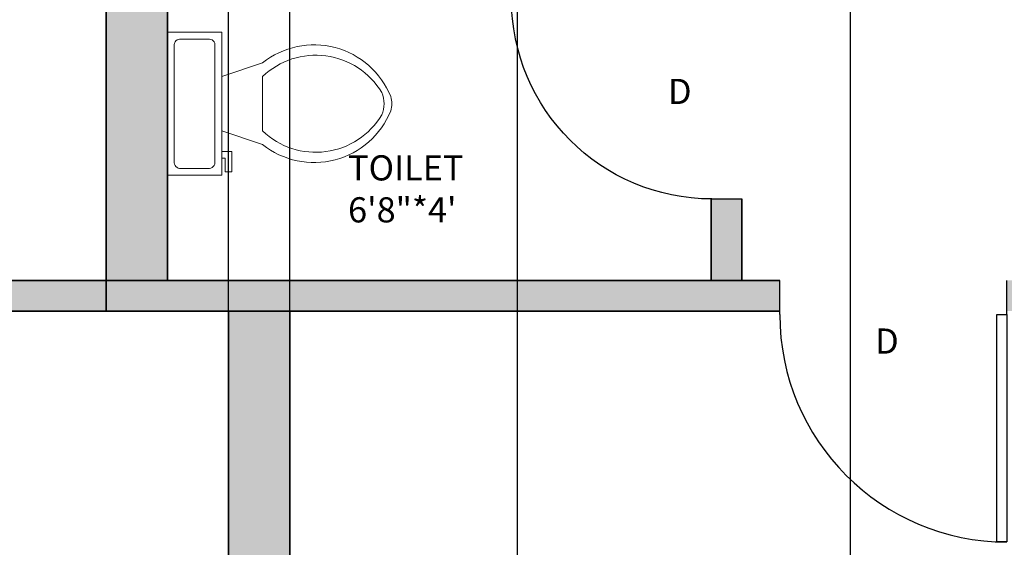
# Model space of a CAD drawing. Units: inches. Extents: x 1998 to 2588, y 1139 to 1977.
# Tile 24 of 134: x 2075 to 2220, y 1668 to 1746. Entities that reach past the tile are written whole.
import ezdxf

# ---------------------------------------------------------------- set-up
doc = ezdxf.new("R2010")
doc.units = ezdxf.units.IN
for name, color, linetype, lineweight in [('A-ANNO-DIMS', 2, 'Continuous', 18), ('A-AREA-IDEN', 7, 'Continuous', 18), ('A-DOOR-IDEN', 7, 'Continuous', 18), ('A-FLOR-FIXT', 9, 'Continuous', 18), ('A-WALL-PATT', 252, 'Continuous', 13), ('DOOR', 52, 'Continuous', 25), ('WALL', 200, 'Continuous', 35)]:
    doc.layers.add(name, color=color, linetype=linetype, lineweight=lineweight)
doc.styles.get("Standard").update_dxf_attribs({"font": 'arial.ttf'})
doc.dimstyles.get("Standard").update_dxf_attribs({"dimtxt": 0.18, "dimasz": 0.18, "dimexe": 0.18, "dimexo": 0.0625, "dimgap": 0.09, "dimtad": 0, "dimtih": 1, "dimtoh": 1, "dimdec": 4, "dimzin": 0, "dimdsep": 46, "dimtxsty": 'Standard', "dimcen": 0.09, "dimadec": 0, "dimazin": 0, "dimtfac": 1, "dimtdec": 4, "dimtofl": 0, "dimtmove": 0, "dimatfit": 3, "dimfxl": 1, "dimtolj": 1, "dimtzin": 0, "dimarcsym": 0})

# ---------------------------------------------------------------- blocks, each defined once
blk = doc.blocks.new('*U2')
for p, q in [((0, 0), (0, -6)), ((40, 0), (40, -6))]:
    blk.add_line(p, q)
blk.add_lwpolyline([(0, 0), (0, 40), (1.75, 40), (1.75, 0)], close=True)
blk.add_arc((0, 0), 40, 0, 90)
blk = doc.blocks.new('*U4')
for p, q in [((9.5, -6), (9.5, -2)), ((-10, -8.5), (-8, -8.5)), ((-10, -9.5), (-10, -8.5)), ((-8, -8.5), (-8, -8)), ((-7, -8), (-7, -9.5)), ((-4, -8), (-6, -14)), ((4, -8), (6, -14)), ((-7, -9.5), (-10, -9.5)), ((4, -14), (-4, -14))]:
    blk.add_line(p, q)
blk.add_lwpolyline([(10.5, -8), (10.5, 0), (-10.5, 0), (-10.5, -8)], close=True)
for points in [[(8.5, -1), (-8.5, -1)], [(-9.5, -2), (-9.5, -6)], [(-8.5, -7), (8.5, -7)]]:
    blk.add_lwpolyline(points)
for centre, radius, start, end in [((-8.62, -1.88), 0.884, 81.8699, 188.1301), ((8.62, -1.88), 0.884, 351.8699, 98.1301), ((-8.62, -6.12), 0.884, 171.8699, 278.1301), ((8.62, -6.12), 0.884, 261.8699, 8.1301), ((3.52, -21.58), 12.17, 141.4691, 247.9714), ((4.2, -21.82), 11.33, 136.3677, 238.9468), ((-3.52, -21.58), 12.17, 292.0284, 38.5307), ((-4.2, -21.82), 11.33, 301.053, 43.6321), ((0, -27.88), 4, 245.7318, 294.2682), ((0, -29), 4, 254.8605, 285.1395)]:
    blk.add_arc(centre, radius, start, end)
blk = doc.blocks.new('*D36')
at = {"layer": 'A-ANNO-DIMS', "color": 0, "lineweight": -2, "transparency": 16777216}
for p, q in [((2197.45, 1663.31), (2197.45, 1977.36)), ((2197.63, 1977.18), (2209.75, 1977.18)), ((2222.79, 1977.18), (2210.68, 1977.18)), ((2222.97, 1663.31), (2222.97, 1977.36))]:
    blk.add_line(p, q, dxfattribs=at)
at = {"layer": 'A-ANNO-DIMS', "color": 0, "transparency": 16777216}
for points in [[(2197.63, 1977.21), (2197.63, 1977.15), (2197.45, 1977.18)], [(2222.79, 1977.21), (2222.79, 1977.15), (2222.97, 1977.18)]]:
    blk.add_solid(points, dxfattribs=at)
at = {"layer": 'Defpoints', "color": 0, "transparency": 16777216}
for p in [(2222.97, 1977.18), (2197.45, 1663.25), (2222.97, 1663.25)]:
    blk.add_point(p, dxfattribs=at)
at = {"layer": 'A-ANNO-DIMS', "color": 0, "transparency": 16777216, "insert": (2210.21, 1977.18), "char_height": 0.18, "attachment_point": 5}
blk.add_mtext('\\A1;25.523', dxfattribs=at)
blk = doc.blocks.new('*D37')
at = {"layer": 'A-ANNO-DIMS', "color": 0, "lineweight": -2, "transparency": 16777216}
for p, q in [((2148.45, 1612.79), (2148.45, 1977.36)), ((2148.63, 1977.18), (2172.73, 1977.18)), ((2197.27, 1977.18), (2173.18, 1977.18)), ((2197.45, 1612.79), (2197.45, 1977.36))]:
    blk.add_line(p, q, dxfattribs=at)
at = {"layer": 'A-ANNO-DIMS', "color": 0, "transparency": 16777216}
for points in [[(2148.63, 1977.21), (2148.63, 1977.15), (2148.45, 1977.18)], [(2197.27, 1977.21), (2197.27, 1977.15), (2197.45, 1977.18)]]:
    blk.add_solid(points, dxfattribs=at)
at = {"layer": 'Defpoints', "color": 0, "transparency": 16777216}
for p in [(2197.45, 1977.18), (2148.45, 1612.73), (2197.45, 1612.73)]:
    blk.add_point(p, dxfattribs=at)
at = {"layer": 'A-ANNO-DIMS', "color": 0, "transparency": 16777216, "insert": (2172.95, 1977.18), "char_height": 0.18, "attachment_point": 5}
blk.add_mtext('\\A1;49', dxfattribs=at)
blk = doc.blocks.new('*D40')
at = {"layer": 'A-ANNO-DIMS', "color": 0, "lineweight": -2, "transparency": 16777216}
for p, q in [((2105.97, 1628.54), (2105.97, 1977.36)), ((2106.15, 1977.18), (2110.32, 1977.18)), ((2114.79, 1977.18), (2110.62, 1977.18)), ((2114.97, 1628.8), (2114.97, 1977.36))]:
    blk.add_line(p, q, dxfattribs=at)
at = {"layer": 'A-ANNO-DIMS', "color": 0, "transparency": 16777216}
for points in [[(2106.15, 1977.21), (2106.15, 1977.15), (2105.97, 1977.18)], [(2114.79, 1977.21), (2114.79, 1977.15), (2114.97, 1977.18)]]:
    blk.add_solid(points, dxfattribs=at)
at = {"layer": 'Defpoints', "color": 0, "transparency": 16777216}
for p in [(2114.97, 1977.18), (2105.97, 1628.48), (2114.97, 1628.74)]:
    blk.add_point(p, dxfattribs=at)
at = {"layer": 'A-ANNO-DIMS', "color": 0, "transparency": 16777216, "insert": (2110.47, 1977.18), "char_height": 0.18, "attachment_point": 5}
blk.add_mtext('\\A1;9', dxfattribs=at)

msp = doc.modelspace()

# ---------------------------------------------------------------- hatches: boundary and pattern name
at = {"layer": 'A-WALL-PATT'}
h = msp.add_hatch(color=256, dxfattribs=at)
h.dxf.hatch_style = 1
h.paths.add_polyline_path([(2222.9729, 1888.7324), (2099.4125, 1888.7324), (2099.4125, 1879.7324), (2222.9729, 1879.7324)])
h.paths.add_polyline_path([(2096.9729, 1868.3278), (2087.9729, 1868.3278), (2087.9729, 1775.637), (2096.9729, 1775.637)])
h.paths.add_polyline_path([(2227.4729, 1868.3278), (2222.9729, 1868.3278), (2222.9729, 1774.3318), (2227.4729, 1774.3318)])
h.paths.add_polyline_path([(2188.3019, 1759.7324), (2138.6074, 1759.7324), (2099.4125, 1759.7324), (2099.4125, 1755.2324), (2176.9729, 1755.2324), (2188.3019, 1755.2324)])
h.paths.add_polyline_path([(2087.9729, 1759.7324), (2059.4729, 1759.7324), (2059.4729, 1702.7324), (2087.9729, 1702.7324), (2087.9729, 1707.2324), (2063.9729, 1707.2324), (2063.9729, 1755.2324), (2087.9729, 1755.2324)])
h.paths.add_polyline_path([(2096.9729, 1755.2324), (2087.9729, 1755.2324), (2087.9729, 1707.2324), (2096.9729, 1707.2324)])
h.paths.add_polyline_path([(2187.0461, 1707.2324), (2105.9729, 1707.2324), (2096.9729, 1707.2324), (2087.9729, 1707.2324), (2087.9729, 1702.7324), (2105.9729, 1702.7324), (2114.9729, 1702.7324), (2187.0461, 1702.7324)])
h.paths.add_polyline_path([(2181.4729, 1719.2028), (2176.9729, 1719.2028), (2176.9729, 1707.2324), (2181.4729, 1707.2324)])
h.paths.add_polyline_path([(2216.0332, 1588.7324), (2114.9729, 1588.7324), (2105.9729, 1588.7324), (2105.9729, 1584.2324), (2216.0332, 1584.2324)])
h.paths.add_polyline_path([(2077.691, 1588.7324), (2061.4729, 1588.7324), (2061.4729, 1584.2324), (2077.691, 1584.2324)])
h.paths.add_polyline_path([(2105.9729, 1588.7324), (2098.0956, 1588.7324), (2098.0956, 1584.2324), (2105.9729, 1584.2324)])
h.paths.add_polyline_path([(2114.9729, 1596.2642), (2110.1012, 1596.2642), (2105.9729, 1596.2642), (2105.9729, 1588.7324), (2114.9729, 1588.7324)])
h.paths.add_polyline_path([(2114.9729, 1584.2324), (2105.9729, 1584.2324), (2105.9729, 1580.249), (2110.1012, 1580.249), (2114.9729, 1580.249)])
h.paths.add_polyline_path([(2114.9729, 1547.7716), (2110.1012, 1547.7716, -0.0318759), (2105.9729, 1548.035), (2105.9729, 1470.2324), (2108.3775, 1470.2324), (2108.3775, 1465.7324), (2186.2943, 1465.7324), (2186.2943, 1470.2324), (2114.9729, 1470.2324)])
h.paths.add_polyline_path([(2227.4729, 1584.2324), (2222.9729, 1584.2324), (2222.9729, 1486.137), (2227.4729, 1486.137)])
h.paths.add_polyline_path([(2295.4138, 1593.2324), (2227.4729, 1593.2324), (2227.4729, 1588.7324), (2295.4138, 1588.7324), (2295.4138, 1591.8729)])
h.paths.add_polyline_path([(2345.9729, 1627.1165), (2341.4729, 1627.1165), (2341.4729, 1593.2324), (2337.2869, 1593.2324), (2337.2869, 1591.8729), (2337.2869, 1588.7324), (2345.9729, 1588.7324)])
h.paths.add_polyline_path([(2291.9729, 1588.7324), (2287.4729, 1588.7324), (2287.4729, 1522.7324), (2291.9729, 1522.7324)])
h.paths.add_polyline_path([(2291.9729, 1522.7324), (2287.4729, 1522.7324), (2227.4729, 1522.7324), (2227.4729, 1518.2324), (2291.9729, 1518.2324)])
h.paths.add_polyline_path([(2295.7347, 1519.5919), (2295.7347, 1522.7324), (2291.9729, 1522.7324), (2291.9729, 1518.2324), (2295.7347, 1518.2324)])
h.paths.add_polyline_path([(2345.9729, 1522.7324), (2337.6078, 1522.7324), (2337.6078, 1519.5919), (2337.6078, 1518.2324), (2341.4729, 1518.2324), (2341.4729, 1488.5616), (2345.9729, 1488.5616)])
h.paths.add_polyline_path([(2345.9729, 1468.1569), (2341.4729, 1468.1569), (2341.4729, 1374.2324), (2227.4729, 1374.2324), (2227.4729, 1369.7324), (2345.9729, 1369.7324)])
h.paths.add_polyline_path([(2345.9729, 1369.7324), (2341.4729, 1369.7324), (2341.4729, 1362.2324), (2345.9729, 1362.2324)])
h.paths.add_polyline_path([(2345.9729, 1317.7324), (2345.9729, 1322.2324), (2341.4729, 1322.2324), (2341.4729, 1285.137), (2345.9729, 1285.137)], flags=17)
h.paths.add_polyline_path([(2356.2096, 1322.2324), (2345.9729, 1322.2324), (2345.9729, 1317.7324), (2356.2096, 1317.7324), (2356.2096, 1319.3088)], flags=17)
h.paths.add_polyline_path([(2393.9729, 1322.2324), (2375.6999, 1322.2324), (2375.6999, 1319.3088, -0.02024576), (2375.636, 1317.7324), (2393.9729, 1317.7324)], flags=17)
h.paths.add_polyline_path([(2398.4729, 1322.2324), (2393.9729, 1322.2324), (2393.9729, 1317.7324), (2393.9729, 1237.7324), (2345.9729, 1237.7324), (2345.9729, 1264.7324), (2341.4729, 1264.7324), (2341.4729, 1228.7324), (2393.9729, 1228.7324), (2482.7412, 1228.7324), (2482.7412, 1237.7324), (2398.4729, 1237.7324), (2398.4729, 1297.1029)])
h.paths.add_polyline_path([(2398.4729, 1362.2324), (2393.9729, 1362.2324), (2393.9729, 1357.7324), (2398.4729, 1357.7324)])
h.paths.add_polyline_path([(2345.9729, 1329.7549), (2341.4729, 1329.7549), (2341.4729, 1322.2324), (2345.9729, 1322.2324)])
h = msp.add_hatch(color=256, dxfattribs=at)
h.dxf.hatch_style = 1
h.paths.add_polyline_path([(2527.4729, 1362.2324), (2510.9729, 1362.2324), (2510.9729, 1357.7324), (2518.4729, 1357.7324), (2518.4729, 1237.7324), (2503.1458, 1237.7324), (2503.1458, 1228.7324), (2527.4729, 1228.7324)])
h.paths.add_polyline_path([(2490.5682, 1362.2324), (2398.4729, 1362.2324), (2398.4729, 1357.7324), (2490.5682, 1357.7324)])
h.paths.add_polyline_path([(2224.9729, 1264.7324), (2222.9729, 1264.7324), (2222.9729, 1232.4125), (2341.4729, 1232.4125), (2341.4729, 1234.4125), (2224.9729, 1234.4125)])
h.paths.add_polyline_path([(2334.5332, 1273.7324), (2264.7638, 1273.7324), (2264.7638, 1269.5611, -0.043659), (2264.3413, 1264.7324), (2334.5332, 1264.7324)])
h.paths.add_polyline_path([(2236.9551, 1273.7324), (2234.4125, 1273.7324), (2234.4125, 1264.7324), (2236.9551, 1264.7324), (2236.9551, 1269.5611)])
h.paths.add_polyline_path([(2222.9729, 1293.2324), (2096.9729, 1293.2324), (2096.9729, 1345.0966), (2087.9729, 1345.0966), (2087.9729, 1284.2324), (2222.9729, 1284.2324), (2222.9729, 1285.137)])
h.paths.add_polyline_path([(2096.9729, 1458.7927), (2087.9729, 1458.7927), (2087.9729, 1417.7324), (2087.9729, 1413.2324), (2096.9729, 1413.2324), (2096.9729, 1417.7324)])
h.paths.add_polyline_path([(2096.9729, 1413.2324), (2087.9729, 1413.2324), (2087.9729, 1365.5012), (2096.9729, 1365.5012), (2096.9729, 1369.3358)])
h.paths.add_polyline_path([(2186.2943, 1417.7324), (2138.6074, 1417.7324), (2096.9729, 1417.7324), (2096.9729, 1413.2324), (2138.6074, 1413.2324), (2186.2943, 1413.2324)])
h.paths.add_polyline_path([(2181.4729, 1465.7324), (2176.9729, 1465.7324), (2176.9729, 1451.6434), (2181.4729, 1451.6434)])
h.paths.add_polyline_path([(2181.4729, 1422.1664), (2176.9729, 1422.1664), (2176.9729, 1417.7324), (2181.4729, 1417.7324)])
h.paths.add_polyline_path([(2063.9729, 1465.7324), (2087.9729, 1465.7324), (2087.9729, 1470.2324), (2059.4729, 1470.2324), (2059.4729, 1413.2324), (2087.9729, 1413.2324), (2087.9729, 1417.7324), (2063.9729, 1417.7324)])
h.paths.add_polyline_path([(2181.4729, 1755.2324), (2176.9729, 1755.2324), (2176.9729, 1748.6798), (2177.0513, 1748.6798), (2181.4729, 1748.6798)])
h.paths.add_polyline_path([(2227.4729, 1707.2324), (2220.4647, 1707.2324), (2220.4647, 1702.7324), (2222.9729, 1702.7324), (2222.9729, 1604.637), (2227.4729, 1604.637)])
h.paths.add_polyline_path([(2114.9729, 1702.7324), (2105.9729, 1702.7324), (2105.9729, 1628.4781, -0.0318759), (2110.1012, 1628.7416), (2114.9729, 1628.7416)])
h.paths.add_polyline_path([(2345.9729, 1739.3278), (2341.4729, 1739.3278), (2341.4729, 1647.5211), (2345.9729, 1647.5211)])
h.paths.add_polyline_path([(2350.6273, 1641.2324), (2345.9729, 1641.2324), (2345.9729, 1636.7324), (2350.6273, 1636.7324), (2350.6273, 1639.8729)])
h.paths.add_polyline_path([(2501.9729, 1641.2324), (2407.9729, 1641.2324), (2392.5005, 1641.2324), (2392.5005, 1639.8729), (2392.5005, 1636.7324), (2501.9729, 1636.7324)])
h.paths.add_polyline_path([(2510.9729, 1755.2324), (2501.9729, 1755.2324), (2501.9729, 1641.2324), (2510.9729, 1641.2324)])
h.paths.add_polyline_path([(2549.1786, 1641.2324), (2522.3775, 1641.2324), (2522.3775, 1636.7324), (2540.1786, 1636.7324), (2540.1786, 1480.7324), (2522.3775, 1480.7324), (2522.3775, 1476.2324), (2549.1786, 1476.2324)])
h.paths.add_polyline_path([(2498.1786, 1594.7324), (2407.9729, 1594.7324), (2407.9729, 1585.7324), (2416.9729, 1585.7324), (2489.1786, 1585.7324), (2489.1786, 1531.7324), (2416.9729, 1531.7324), (2407.9729, 1531.7324), (2407.9729, 1522.7324), (2498.1786, 1522.7324)])
h.paths.add_polyline_path([(2351.6437, 1480.7324), (2345.9729, 1480.7324), (2345.9729, 1476.2324), (2351.6437, 1476.2324), (2351.6437, 1477.5919)])
h.paths.add_polyline_path([(2501.9729, 1480.7324), (2498.1786, 1480.7324), (2407.9729, 1480.7324), (2393.5168, 1480.7324), (2393.5168, 1477.5919), (2393.5168, 1476.2324), (2501.9729, 1476.2324)])

# ---------------------------------------------------------------- linework, layer by layer
at = {"layer": 'WALL'}
for p, q in [((2087.9729, 1755.2324), (2087.9729, 1702.7324)), ((2096.9729, 1755.2324), (2096.9729, 1707.2324)), ((2176.9729, 1719.2029), (2176.9729, 1707.2324)), ((2181.4729, 1719.2028), (2181.4729, 1707.2324)), ((2063.9729, 1707.2324), (2087.9729, 1707.2324)), ((2081.9729, 1707.2324), (2114.9729, 1707.2324)), ((2096.9729, 1707.2324), (2105.9729, 1707.2324)), ((2096.9729, 1707.2324), (2176.9729, 1707.2324)), ((2187.0461, 1707.2324), (2105.9729, 1707.2324)), ((2187.0461, 1707.2324), (2114.9729, 1707.2324)), ((2059.4729, 1702.7324), (2087.9729, 1702.7324)), ((2077.4729, 1702.7324), (2114.9729, 1702.7324)), ((2105.9729, 1702.7324), (2087.9729, 1702.7324)), ((2187.0461, 1702.7324), (2105.9729, 1702.7324)), ((2105.9729, 1628.4781), (2105.9729, 1702.7324)), ((2187.0461, 1702.7324), (2114.9729, 1702.7324)), ((2114.9729, 1628.7416), (2114.9729, 1702.7324))]:
    msp.add_line(p, q, dxfattribs=at)

# ---------------------------------------------------------------- block references
at = {"layer": 'A-FLOR-FIXT', "rotation": 90.00000000000003}
msp.add_blockref('*U4', (2096.9729, 1733.1987), dxfattribs=at)
at = {"layer": 'DOOR'}
for p, xscale, yscale, zscale, rotation in [((2177.0513, 1748.6798), -0.736924595324625, 0.736924595324625, 0.736924595324625, 90), ((2220.4647, 1702.2196), 0.8354643497673233, 0.8354643497673233, 0.8354643497673233, 180)]:
    msp.add_blockref('*U2', p, dxfattribs=dict(at, xscale=xscale, yscale=yscale, zscale=zscale, rotation=rotation))

# ---------------------------------------------------------------- texts
at = {"layer": 'A-AREA-IDEN', "insert": (2123.5492, 1725.622), "char_height": 3.69875, "attachment_point": 1}
msp.add_mtext_dynamic_manual_height_columns('TOILET\\P6\'8"*4\'', width=110.572713, gutter_width=18.4938, heights=[0], dxfattribs=at)
at = {"layer": 'A-DOOR-IDEN', "char_height": 3.6988, "attachment_point": 1}
for insert in [(2170.6122, 1736.8545), (2201.0808, 1700.1723)]:
    msp.add_mtext_dynamic_manual_height_columns('D', width=110.572713, gutter_width=18.4938, heights=[0], dxfattribs=dict(at, insert=insert))

# ---------------------------------------------------------------- dimensions: what is measured, and where the dimension line sits
at = {"layer": 'A-ANNO-DIMS'}
for base, p1, p2, override, picture, middle in [((2114.9729, 1977.1824), (2105.9729, 1628.4781), (2114.9729, 1628.7416), {"dimdec": 0, "dimlfac": 1, "dimrnd": 0, "dimzin": 0, "dimdsep": 46, "dimlunit": 2}, '*D40', (2110.4729, 1977.1824)), ((2197.4499, 1977.1824), (2148.4548, 1612.7324), (2197.4499, 1612.7324), {"dimdec": 0, "dimlfac": 1, "dimrnd": 0, "dimzin": 0, "dimdsep": 46, "dimlunit": 2}, '*D37', (2172.9524, 1977.1824)), ((2222.9729, 1977.1824), (2197.4499, 1663.2466), (2222.9729, 1663.2466), {"dimdec": 3, "dimlfac": 1, "dimrnd": 0, "dimzin": 0, "dimdsep": 46, "dimlunit": 2}, '*D36', (2210.2114, 1977.1824))]:
    dim = msp.add_linear_dim(base=base, p1=p1, p2=p2, dimstyle='Standard', override=override, dxfattribs=at)
    dim.commit()
    dim.dimension.update_dxf_attribs({"geometry": picture, "text_midpoint": middle})

doc.saveas('drawing.dxf')
